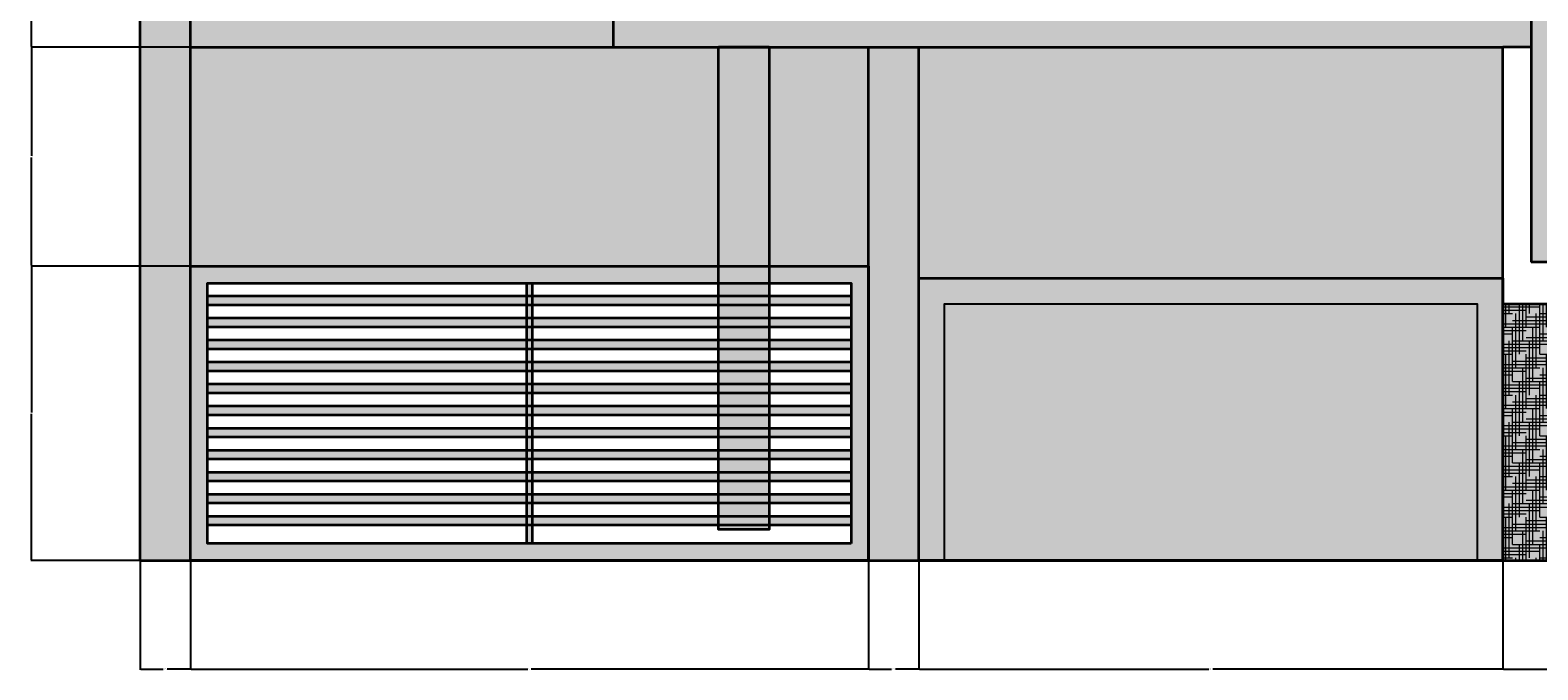
# Model space of a CAD drawing. Units: feet. Extents: x 2415 to 6174, y 866 to 1295.
# Tile 1 of 9: x 3227 to 3580, y 866 to 1016. Entities that reach past the tile are written whole.
import ezdxf

# ---------------------------------------------------------------- set-up
doc = ezdxf.new("R2010")
doc.units = ezdxf.units.FT
for name, color, linetype, lineweight in [('A-ANNO-DIMS', 2, 'Continuous', 18), ('A-DOOR', 4, 'Continuous', 25), ('A-ELEV', 7, 'Continuous', 35), ('A-ELEV-PATT', 8, 'Continuous', 13)]:
    doc.layers.add(name, color=color, linetype=linetype, lineweight=lineweight)
doc.styles.get("Standard").update_dxf_attribs({"font": 'arial.ttf'})
doc.dimstyles.get("Standard").update_dxf_attribs({"dimtxt": 0.18, "dimasz": 0.18, "dimexe": 0.18, "dimexo": 0.0625, "dimgap": 0.09, "dimtad": 0, "dimtih": 1, "dimtoh": 1, "dimdec": 1, "dimzin": 0, "dimdsep": 46, "dimlunit": 3, "dimtxsty": 'Standard', "dimcen": 0.09, "dimadec": 0, "dimazin": 0, "dimtfac": 1, "dimtdec": 1, "dimtofl": 0, "dimtmove": 0, "dimatfit": 3, "dimfxl": 1, "dimtolj": 1, "dimtzin": 0, "dimarcsym": 0})

# ---------------------------------------------------------------- blocks, each defined once
blk = doc.blocks.new('GATE-MAIN')
blk.add_line((0, 60), (124.63, 60))
for points in [[(0, 0), (0, 60)], [(124.63, 60), (124.63, 0)]]:
    blk.add_lwpolyline(points)
blk.add_lwpolyline([(124.63, 0), (0, 0), (0, 60), (124.63, 60)], close=True)
blk = doc.blocks.new('*D53')
at = {"layer": 'A-ANNO-DIMS', "color": 0, "lineweight": -2, "transparency": 16777216}
for p, q in [((3253.13, 891.54), (3253.13, 866.02)), ((3264.92, 891.54), (3264.92, 866.02)), ((3253.31, 866.2), (3258.57, 866.2)), ((3264.74, 866.2), (3259.48, 866.2))]:
    blk.add_line(p, q, dxfattribs=at)
at = {"layer": 'A-ANNO-DIMS', "color": 0, "transparency": 16777216}
for points in [[(3253.31, 866.23), (3253.31, 866.17), (3253.13, 866.2)], [(3264.74, 866.23), (3264.74, 866.17), (3264.92, 866.2)]]:
    blk.add_solid(points, dxfattribs=at)
at = {"layer": 'Defpoints', "color": 0, "transparency": 16777216}
for p in [(3253.13, 891.6), (3264.92, 891.6), (3264.92, 866.2)]:
    blk.add_point(p, dxfattribs=at)
at = {"layer": 'A-ANNO-DIMS', "color": 0, "transparency": 16777216, "insert": (3259.02, 866.2), "char_height": 0.18, "attachment_point": 5}
blk.add_mtext('\\A1;11.787', dxfattribs=at)
blk = doc.blocks.new('*D54')
at = {"layer": 'A-ANNO-DIMS', "color": 0, "lineweight": -2, "transparency": 16777216}
for p, q in [((3264.92, 891.54), (3264.92, 866.02)), ((3423.52, 891.54), (3423.52, 866.02)), ((3265.1, 866.2), (3343.83, 866.2)), ((3423.34, 866.2), (3344.6, 866.2))]:
    blk.add_line(p, q, dxfattribs=at)
at = {"layer": 'A-ANNO-DIMS', "color": 0, "transparency": 16777216}
for points in [[(3265.1, 866.23), (3265.1, 866.17), (3264.92, 866.2)], [(3423.34, 866.23), (3423.34, 866.17), (3423.52, 866.2)]]:
    blk.add_solid(points, dxfattribs=at)
at = {"layer": 'Defpoints', "color": 0, "transparency": 16777216}
for p in [(3264.92, 891.6), (3423.52, 891.6), (3423.52, 866.2)]:
    blk.add_point(p, dxfattribs=at)
at = {"layer": 'A-ANNO-DIMS', "color": 0, "transparency": 16777216, "insert": (3344.22, 866.2), "char_height": 0.18, "attachment_point": 5}
blk.add_mtext('\\A1;158.6', dxfattribs=at)
blk = doc.blocks.new('*D55')
at = {"layer": 'A-ANNO-DIMS', "color": 0, "lineweight": -2, "transparency": 16777216}
for p, q in [((3423.52, 891.54), (3423.52, 866.02)), ((3435.31, 891.54), (3435.31, 866.02)), ((3423.7, 866.2), (3428.96, 866.2)), ((3435.13, 866.2), (3429.87, 866.2))]:
    blk.add_line(p, q, dxfattribs=at)
at = {"layer": 'A-ANNO-DIMS', "color": 0, "transparency": 16777216}
for points in [[(3423.7, 866.23), (3423.7, 866.17), (3423.52, 866.2)], [(3435.13, 866.23), (3435.13, 866.17), (3435.31, 866.2)]]:
    blk.add_solid(points, dxfattribs=at)
at = {"layer": 'Defpoints', "color": 0, "transparency": 16777216}
for p in [(3423.52, 891.6), (3435.31, 891.6), (3435.31, 866.2)]:
    blk.add_point(p, dxfattribs=at)
at = {"layer": 'A-ANNO-DIMS', "color": 0, "transparency": 16777216, "insert": (3429.41, 866.2), "char_height": 0.18, "attachment_point": 5}
blk.add_mtext('\\A1;11.787', dxfattribs=at)
blk = doc.blocks.new('*D56')
at = {"layer": 'A-ANNO-DIMS', "color": 0, "lineweight": -2, "transparency": 16777216}
for p, q in [((3435.31, 891.54), (3435.31, 866.02)), ((3571.93, 891.54), (3571.93, 866.02)), ((3435.49, 866.2), (3503.17, 866.2)), ((3571.75, 866.2), (3504.08, 866.2))]:
    blk.add_line(p, q, dxfattribs=at)
at = {"layer": 'A-ANNO-DIMS', "color": 0, "transparency": 16777216}
for points in [[(3435.49, 866.23), (3435.49, 866.17), (3435.31, 866.2)], [(3571.75, 866.23), (3571.75, 866.17), (3571.93, 866.2)]]:
    blk.add_solid(points, dxfattribs=at)
at = {"layer": 'Defpoints', "color": 0, "transparency": 16777216}
for p in [(3435.31, 891.6), (3571.93, 891.6), (3571.93, 866.2)]:
    blk.add_point(p, dxfattribs=at)
at = {"layer": 'A-ANNO-DIMS', "color": 0, "transparency": 16777216, "insert": (3503.62, 866.2), "char_height": 0.18, "attachment_point": 5}
blk.add_mtext('\\A1;136.63', dxfattribs=at)
blk = doc.blocks.new('*D57')
at = {"layer": 'A-ANNO-DIMS', "color": 0, "lineweight": -2, "transparency": 16777216}
for p, q in [((3571.93, 891.54), (3571.93, 866.02)), ((3601, 891.54), (3601, 866.02)), ((3572.11, 866.2), (3586.07, 866.2)), ((3600.82, 866.2), (3586.86, 866.2))]:
    blk.add_line(p, q, dxfattribs=at)
at = {"layer": 'A-ANNO-DIMS', "color": 0, "transparency": 16777216}
for points in [[(3572.11, 866.23), (3572.11, 866.17), (3571.93, 866.2)], [(3600.82, 866.23), (3600.82, 866.17), (3601, 866.2)]]:
    blk.add_solid(points, dxfattribs=at)
at = {"layer": 'Defpoints', "color": 0, "transparency": 16777216}
for p in [(3571.93, 891.6), (3601, 891.6), (3601, 866.2)]:
    blk.add_point(p, dxfattribs=at)
at = {"layer": 'A-ANNO-DIMS', "color": 0, "transparency": 16777216, "insert": (3586.47, 866.2), "char_height": 0.18, "attachment_point": 5}
blk.add_mtext('\\A1;29.06', dxfattribs=at)
blk = doc.blocks.new('*D72')
at = {"layer": 'A-ANNO-DIMS', "color": 0, "lineweight": -2, "transparency": 16777216}
for p, q in [((3264.85, 960.43), (3227.55, 960.43)), ((3227.73, 960.25), (3227.73, 926.2)), ((3227.73, 891.78), (3227.73, 925.83)), ((3264.85, 891.6), (3227.55, 891.6))]:
    blk.add_line(p, q, dxfattribs=at)
at = {"layer": 'A-ANNO-DIMS', "color": 0, "transparency": 16777216}
for points in [[(3227.7, 960.25), (3227.76, 960.25), (3227.73, 960.43)], [(3227.7, 891.78), (3227.76, 891.78), (3227.73, 891.6)]]:
    blk.add_solid(points, dxfattribs=at)
at = {"layer": 'Defpoints', "color": 0, "transparency": 16777216}
for p in [(3227.73, 960.43), (3264.92, 960.43), (3264.92, 891.6)]:
    blk.add_point(p, dxfattribs=at)
at = {"layer": 'A-ANNO-DIMS', "color": 0, "transparency": 16777216, "insert": (3227.73, 926.02), "char_height": 0.18, "attachment_point": 5}
blk.add_mtext('\\A1;68.83', dxfattribs=at)
blk = doc.blocks.new('*D73')
at = {"layer": 'A-ANNO-DIMS', "color": 0, "lineweight": -2, "transparency": 16777216}
for p, q in [((3264.85, 1011.6), (3227.55, 1011.6)), ((3227.73, 1011.42), (3227.73, 986.2)), ((3227.73, 960.61), (3227.73, 985.83)), ((3264.85, 960.43), (3227.55, 960.43))]:
    blk.add_line(p, q, dxfattribs=at)
at = {"layer": 'A-ANNO-DIMS', "color": 0, "transparency": 16777216}
for points in [[(3227.7, 1011.42), (3227.76, 1011.42), (3227.73, 1011.6)], [(3227.7, 960.61), (3227.76, 960.61), (3227.73, 960.43)]]:
    blk.add_solid(points, dxfattribs=at)
at = {"layer": 'Defpoints', "color": 0, "transparency": 16777216}
for p in [(3227.73, 1011.6), (3264.92, 1011.6), (3264.92, 960.43)]:
    blk.add_point(p, dxfattribs=at)
at = {"layer": 'A-ANNO-DIMS', "color": 0, "transparency": 16777216, "insert": (3227.73, 986.02), "char_height": 0.18, "attachment_point": 5}
blk.add_mtext('\\A1;51.17', dxfattribs=at)
blk = doc.blocks.new('*D74')
at = {"layer": 'A-ANNO-DIMS', "color": 0, "lineweight": -2, "transparency": 16777216}
for p, q in [((3288.28, 1042.32), (3227.55, 1042.32)), ((3227.73, 1042.14), (3227.73, 1027.14)), ((3227.73, 1011.78), (3227.73, 1026.78)), ((3264.85, 1011.6), (3227.55, 1011.6))]:
    blk.add_line(p, q, dxfattribs=at)
at = {"layer": 'A-ANNO-DIMS', "color": 0, "transparency": 16777216}
for points in [[(3227.7, 1042.14), (3227.76, 1042.14), (3227.73, 1042.32)], [(3227.7, 1011.78), (3227.76, 1011.78), (3227.73, 1011.6)]]:
    blk.add_solid(points, dxfattribs=at)
at = {"layer": 'Defpoints', "color": 0, "transparency": 16777216}
for p in [(3227.73, 1042.32), (3288.35, 1042.32), (3264.92, 1011.6)]:
    blk.add_point(p, dxfattribs=at)
at = {"layer": 'A-ANNO-DIMS', "color": 0, "transparency": 16777216, "insert": (3227.73, 1026.96), "char_height": 0.18, "attachment_point": 5}
blk.add_mtext('\\A1;30.72', dxfattribs=at)

msp = doc.modelspace()

# ---------------------------------------------------------------- hatches: boundary and pattern name
at = {"layer": 'A-ELEV-PATT'}
h = msp.add_hatch(color=256, dxfattribs=at)
h.set_gradient(color1=(255, 255, 255), tint=1)
h.paths.add_polyline_path([(3264.916, 1143.5993), (3253.129, 1143.5993), (3253.129, 891.5992), (3264.916, 891.5992)])
h.paths.add_polyline_path([(3470.0448, 1143.5993), (3264.916, 1143.5993), (3264.916, 1137.5993), (3466.5999, 1137.5993)])
h.paths.add_polyline_path([(3363.8667, 1137.5993), (3264.916, 1137.5993), (3264.916, 1011.5992), (3363.8667, 1011.5992)])
h.paths.add_polyline_path([(3286.0429, 1117.0591), (3337.7904, 1117.0591), (3337.7904, 1115.4381), (3336.5314, 1115.4381), (3336.5314, 1110.528), (3335.4882, 1110.528), (3335.4882, 1042.3194), (3288.3452, 1042.3194), (3288.3452, 1110.528), (3287.3019, 1110.528), (3287.3019, 1115.4381), (3286.0429, 1115.4381)], flags=16)
h.paths.add_polyline_path([(3290.3452, 1108.528), (3333.4882, 1108.528), (3333.4882, 1044.3194), (3290.3452, 1044.3194)], flags=0)
h.paths.add_polyline_path([(3292.3452, 1106.528), (3331.4882, 1106.528), (3331.4882, 1046.3194), (3292.3452, 1046.3194)], flags=0)
h.paths.add_polyline_path([(3311.7156, 1106.528), (3312.1178, 1106.528), (3312.1178, 1046.3194), (3311.7156, 1046.3194)], flags=0)
h.paths.add_polyline_path([(3682.0722, 1263.5993), (3578.5579, 1263.5993), (3578.5579, 1137.5993), (3578.5579, 961.3655), (3682.0722, 961.3655)])
h.paths.add_polyline_path([(3660.8129, 1239.0671), (3660.8129, 996.6447), (3602.2151, 996.6447), (3602.2151, 1239.0671)], flags=16)
h.paths.add_polyline_path([(3632.2447, 1239.0671), (3632.2447, 996.6447), (3630.7833, 996.6447), (3630.7833, 1029.3019), (3602.2151, 1029.3019), (3602.2151, 1030.7632), (3630.7833, 1030.7632), (3630.7833, 1071.2549), (3602.2151, 1071.2549), (3602.2151, 1072.7163), (3630.7833, 1072.7163), (3630.7833, 1113.2079), (3602.2151, 1113.2079), (3602.2151, 1114.6693), (3630.7833, 1114.6693), (3630.7833, 1155.161), (3602.2151, 1155.161), (3602.2151, 1156.6224), (3630.7833, 1156.6224), (3630.7833, 1197.114), (3602.2151, 1197.114), (3602.2151, 1198.5754), (3630.7833, 1198.5754), (3630.7833, 1239.0671)], flags=0)
h.paths.add_polyline_path([(3733.129, 951.5993), (3634.5374, 951.5993), (3634.5374, 891.5992), (3733.129, 891.5992)])
h.paths.add_polyline_path([(3627.8799, 951.5993), (3621.0953, 951.5993), (3621.0953, 891.5992), (3627.8799, 891.5992)])
h.paths.add_polyline_path([(3614.4378, 951.5993), (3607.6532, 951.5993), (3607.6532, 891.5992), (3614.4378, 891.5992)])
h.paths.add_polyline_path([(3565.9347, 951.5993), (3441.3079, 951.5993), (3441.3079, 891.5992), (3565.9347, 891.5992)], flags=17)
h.paths.add_polyline_path([(3571.9347, 957.5993), (3435.3079, 957.5993), (3435.3079, 891.5992), (3441.3079, 891.5992), (3441.3079, 951.5993), (3565.9347, 951.5993), (3565.9347, 891.5992), (3571.9347, 891.5992)])
h.paths.add_polyline_path([(3435.3079, 1011.5992), (3423.5209, 1011.5992), (3423.5209, 891.5992), (3435.3079, 891.5992), (3435.3079, 957.5993)])
h.paths.add_polyline_path([(3690.0912, 1269.5993), (3571.9347, 1269.5993), (3571.9347, 1263.5993), (3690.0912, 1263.5993)])
h.paths.add_polyline_path([(3571.9347, 1269.5993), (3538.5122, 1257.6449), (3538.5122, 1251.6449), (3571.9347, 1263.5993)])
h = msp.add_hatch(color=256, dxfattribs=at)
h.set_gradient(color1=(99, 100, 102), color2=(99, 100, 102))
h.paths.add_polyline_path([(3578.5579, 1137.5993), (3363.8667, 1137.5993), (3363.8667, 1123.5993), (3371.8667, 1123.5993), (3371.8667, 1129.5993), (3570.5579, 1129.5993), (3570.5579, 1019.5993), (3371.8667, 1019.5993), (3371.8667, 1027.963), (3363.8667, 1027.963), (3363.8667, 1011.5992), (3571.9347, 1011.5992), (3578.5579, 1011.5992)])
h.paths.add_polyline_path([(3371.8667, 1123.5993), (3363.8667, 1123.5993), (3363.8667, 1053.4585), (3371.8667, 1053.4585)], flags=17)
h.paths.add_polyline_path([(3371.8667, 1042.1234), (3363.8667, 1042.1234), (3363.8667, 1028.2269), (3371.8667, 1028.2269)], flags=17)
h.paths.add_polyline_path([(3371.8667, 1051.7117), (3363.8667, 1051.7117), (3363.8667, 1042.3873), (3371.8667, 1042.3873)], flags=17)
h.paths.add_polyline_path([(3371.8667, 1053.4585), (3363.8667, 1053.4585), (3363.8667, 1051.7117), (3371.8667, 1051.7117)], flags=17)
h.paths.add_polyline_path([(3371.8667, 1042.3873), (3363.8667, 1042.3873), (3363.8667, 1042.1234), (3371.8667, 1042.1234)], flags=17)
h.paths.add_polyline_path([(3371.8667, 1028.2269), (3363.8667, 1028.2269), (3363.8667, 1027.963), (3371.8667, 1027.963)], flags=17)
h = msp.add_hatch(color=256, dxfattribs=at)
h.set_gradient(color1=(248, 246, 176), name='CURVED')
h.paths.add_polyline_path([(3487.443, 1123.5993), (3446.1534, 1123.5993), (3446.1534, 1053.4585), (3487.443, 1053.4585), (3487.443, 1080.8275)])
h.paths.add_polyline_path([(3468.3641, 1051.7117), (3446.1534, 1051.7117), (3446.1534, 1028.2269), (3468.3641, 1028.2269)])
h.paths.add_polyline_path([(3487.443, 1051.7117), (3468.628, 1051.7117), (3468.628, 1028.2269), (3487.443, 1028.2269)])
h.paths.add_polyline_path([(3468.3641, 1027.963), (3446.1534, 1027.963), (3446.1534, 1019.5993), (3468.3641, 1019.5993)])
h.paths.add_polyline_path([(3487.443, 1027.963), (3468.628, 1027.963), (3468.628, 1019.5993), (3487.443, 1019.5993)])
h.paths.add_polyline_path([(3564.5579, 1123.5993), (3530.9457, 1099.6515), (3487.443, 1099.6515), (3487.443, 1080.8275), (3524.8012, 1080.8275), (3524.8012, 1053.4585), (3564.5579, 1053.4585)])
h.paths.add_polyline_path([(3548.7638, 1051.7117), (3524.8012, 1051.7117), (3524.8012, 1028.2269), (3548.7638, 1028.2269)])
h.paths.add_polyline_path([(3548.7638, 1027.963), (3524.8012, 1027.963), (3524.8012, 1019.5993), (3548.7638, 1019.5993)])
h.paths.add_polyline_path([(3564.5579, 1027.963), (3549.0277, 1027.963), (3549.0277, 1019.5993), (3564.5579, 1019.5993)])
h.paths.add_polyline_path([(3388.4421, 1011.5992), (3264.916, 1011.5992), (3264.916, 960.433), (3388.4421, 960.433)])
h.paths.add_polyline_path([(3571.9347, 1011.5992), (3435.3079, 1011.5992), (3435.3079, 957.5993), (3571.9347, 957.5993)])
h.paths.add_polyline_path([(3423.5209, 1011.5992), (3400.3333, 1011.5992), (3400.3333, 960.433), (3423.5209, 960.433)])
h = msp.add_hatch(color=256, dxfattribs=at)
h.set_gradient(color1=(203, 74, 40), color2=(203, 74, 40))
h.paths.add_polyline_path([(3400.3333, 1011.5992), (3388.4421, 1011.5992), (3388.4421, 960.433), (3400.3333, 960.433)])
h.paths.add_polyline_path([(3400.3333, 956.433), (3388.4421, 956.433), (3388.4421, 953.4503), (3400.3333, 953.4503)])
h.paths.add_polyline_path([(3400.3333, 951.2861), (3388.4421, 951.2861), (3388.4421, 948.3033), (3400.3333, 948.3033)])
h.paths.add_polyline_path([(3400.3333, 946.1391), (3388.4421, 946.1391), (3388.4421, 943.1563), (3400.3333, 943.1563)])
h.paths.add_polyline_path([(3400.3333, 940.9922), (3388.4421, 940.9922), (3388.4421, 938.0094), (3400.3333, 938.0094)])
h.paths.add_polyline_path([(3400.3333, 935.8452), (3388.4421, 935.8452), (3388.4421, 932.8624), (3400.3333, 932.8624)])
h.paths.add_polyline_path([(3400.3333, 930.6983), (3388.4421, 930.6983), (3388.4421, 927.7155), (3400.3333, 927.7155)])
h.paths.add_polyline_path([(3400.3333, 925.5513), (3388.4421, 925.5513), (3388.4421, 922.5685), (3400.3333, 922.5685)])
h.paths.add_polyline_path([(3400.3333, 920.4043), (3388.4421, 920.4043), (3388.4421, 917.4215), (3400.3333, 917.4215)])
h.paths.add_polyline_path([(3400.3333, 915.2574), (3388.4421, 915.2574), (3388.4421, 912.2746), (3400.3333, 912.2746)])
h.paths.add_polyline_path([(3400.3333, 910.1104), (3388.4421, 910.1104), (3388.4421, 907.1276), (3400.3333, 907.1276)])
h.paths.add_polyline_path([(3400.3333, 904.9635), (3388.4421, 904.9635), (3388.4421, 901.9807), (3400.3333, 901.9807)])
h.paths.add_polyline_path([(3400.3333, 899.8165), (3388.4421, 899.8165), (3388.4421, 898.815), (3400.3333, 898.815)])
h = msp.add_hatch(color=256, dxfattribs=at)
h.set_gradient(color1=(248, 246, 176), color2=(248, 246, 176), name='CURVED')
h.paths.add_polyline_path([(3571.9347, 1011.5992), (3435.3079, 1011.5992), (3435.3079, 957.5993), (3571.9347, 957.5993)])
h = msp.add_hatch(color=256, dxfattribs=at)
h.set_gradient(color1=(147, 149, 152), color2=(99, 100, 102))
h.paths.add_polyline_path([(3423.523, 960.4469), (3264.9181, 960.4469), (3264.9181, 891.6131), (3423.523, 891.6131)])
h.paths.add_polyline_path([(3268.9181, 956.4469), (3419.523, 956.4469), (3419.523, 895.6131), (3268.9181, 895.6131)], flags=16)
h.paths.add_polyline_path([(3268.9181, 953.4641), (3343.5898, 953.4641), (3343.5898, 956.4469), (3344.8513, 956.4469), (3344.8513, 953.4641), (3419.523, 953.4641), (3419.523, 951.2999), (3344.8513, 951.2999), (3344.8513, 948.3172), (3419.523, 948.3172), (3419.523, 946.153), (3344.8513, 946.153), (3344.8513, 943.1702), (3419.523, 943.1702), (3419.523, 941.006), (3344.8513, 941.006), (3344.8513, 938.0232), (3419.523, 938.0232), (3419.523, 935.8591), (3344.8513, 935.8591), (3344.8513, 932.8763), (3419.523, 932.8763), (3419.523, 930.7121), (3344.8513, 930.7121), (3344.8513, 927.7293), (3419.523, 927.7293), (3419.523, 925.5652), (3344.8513, 925.5652), (3344.8513, 922.5824), (3419.523, 922.5824), (3419.523, 920.4182), (3344.8513, 920.4182), (3344.8513, 917.4354), (3419.523, 917.4354), (3419.523, 915.2712), (3344.8513, 915.2712), (3344.8513, 912.2884), (3419.523, 912.2884), (3419.523, 910.1243), (3344.8513, 910.1243), (3344.8513, 907.1415), (3419.523, 907.1415), (3419.523, 904.9773), (3344.8513, 904.9773), (3344.8513, 901.9945), (3419.523, 901.9945), (3419.523, 899.8304), (3344.8513, 899.8304), (3344.8513, 895.6131), (3343.5898, 895.6131), (3343.5898, 899.8304), (3268.9181, 899.8304), (3268.9181, 901.9945), (3343.5898, 901.9945), (3343.5898, 904.9773), (3268.9181, 904.9773), (3268.9181, 907.1415), (3343.5898, 907.1415), (3343.5898, 910.1243), (3268.9181, 910.1243), (3268.9181, 912.2884), (3343.5898, 912.2884), (3343.5898, 915.2712), (3268.9181, 915.2712), (3268.9181, 917.4354), (3343.5898, 917.4354), (3343.5898, 920.4182), (3268.9181, 920.4182), (3268.9181, 922.5824), (3343.5898, 922.5824), (3343.5898, 925.5652), (3268.9181, 925.5652), (3268.9181, 927.7293), (3343.5898, 927.7293), (3343.5898, 930.7121), (3268.9181, 930.7121), (3268.9181, 932.8763), (3343.5898, 932.8763), (3343.5898, 935.8591), (3268.9181, 935.8591), (3268.9181, 938.0232), (3343.5898, 938.0232), (3343.5898, 941.006), (3268.9181, 941.006), (3268.9181, 943.1702), (3343.5898, 943.1702), (3343.5898, 946.153), (3268.9181, 946.153), (3268.9181, 948.3172), (3343.5898, 948.3172), (3343.5898, 951.2999), (3268.9181, 951.2999)], flags=16)
h = msp.add_hatch(color=256, dxfattribs=at)
h.set_gradient(color1=(99, 100, 102), color2=(99, 100, 102))
h.paths.add_polyline_path([(3607.6532, 957.5993), (3600.9957, 957.5993), (3600.9957, 891.5992), (3607.6532, 891.5992)])
h.paths.add_polyline_path([(3621.0953, 957.5993), (3614.4378, 957.5993), (3614.4378, 891.5992), (3621.0953, 891.5992)])
h.paths.add_polyline_path([(3634.5374, 957.5993), (3627.8799, 957.5993), (3627.8799, 891.5992), (3634.5374, 891.5992)])
h.paths.add_polyline_path([(3600.9957, 951.5993), (3571.9347, 951.5993), (3571.9347, 891.5992), (3600.9957, 891.5992)])
h = msp.add_hatch(dxfattribs=at)
h.set_pattern_fill('HOUND', color=256, scale=0.5, style=0)
h.set_pattern_definition([(0, (850.0754, 0), (3.175, 0.79375), [12.7, -6.35]), (90, (850.0754, 0), (-0.79375, -3.175), [12.7, -6.35])])
h.paths.add_polyline_path([(3607.6532, 957.5993), (3600.9957, 957.5993), (3600.9957, 891.5992), (3607.6532, 891.5992)])
h.paths.add_polyline_path([(3621.0953, 957.5993), (3614.4378, 957.5993), (3614.4378, 891.5992), (3621.0953, 891.5992)])
h.paths.add_polyline_path([(3634.5374, 957.5993), (3627.8799, 957.5993), (3627.8799, 891.5992), (3634.5374, 891.5992)])
h.paths.add_polyline_path([(3600.9957, 951.5993), (3571.9347, 951.5993), (3571.9347, 891.5992), (3600.9957, 891.5992)])

# ---------------------------------------------------------------- linework, layer by layer
at = {"layer": 'A-ELEV'}
for p, q in [((3253.129, 891.5992), (3253.129, 1143.5993)), ((3363.8667, 1011.5992), (3363.8667, 1137.5993)), ((3578.5579, 1137.5993), (3578.5579, 961.3655)), ((3264.916, 1011.5992), (3571.9347, 1011.5992)), ((3423.5209, 891.5992), (3423.5209, 1011.5992)), ((3435.3079, 891.5992), (3435.3079, 1011.5992)), ((3571.9347, 891.5992), (3571.9347, 1011.5992)), ((3435.3079, 957.5993), (3571.9347, 957.5993)), ((3571.9347, 951.5993), (3600.9957, 951.5993)), ((3253.129, 891.5992), (3733.129, 891.5992))]:
    msp.add_line(p, q, dxfattribs=at)
for points in [[(3682.0722, 1263.5993), (3682.0722, 961.3655), (3578.5579, 961.3655)], [(3253.129, 891.5992), (3264.916, 891.5992), (3264.916, 1143.5993)], [(3578.5579, 1137.5993), (3578.5579, 1137.5993), (3578.5579, 1011.5992), (3571.9347, 1011.5992)], [(3400.3333, 1011.5992), (3388.4421, 1011.5992)], [(3400.3333, 1011.5992), (3400.3333, 898.815), (3388.4421, 898.815), (3388.4421, 1011.5992)], [(3423.5209, 891.5992), (3435.3079, 891.5992)], [(3571.9347, 891.5992), (3435.3079, 891.5992)]]:
    msp.add_lwpolyline(points, dxfattribs=at)
for points in [[(3423.5209, 891.5992), (3264.916, 891.5992), (3264.916, 960.433), (3423.5209, 960.433)], [(3419.5209, 895.5993), (3268.916, 895.5993), (3268.916, 956.433), (3419.5209, 956.433)], [(3343.5877, 956.433), (3344.8492, 956.433), (3344.8492, 895.5993), (3343.5877, 895.5993)], [(3571.9347, 891.5992), (3435.3079, 891.5992), (3435.3079, 957.5993), (3571.9347, 957.5993)], [(3268.916, 953.4503), (3419.5209, 953.4503), (3419.5209, 951.2861), (3268.916, 951.2861)], [(3268.916, 948.3033), (3419.5209, 948.3033), (3419.5209, 946.1391), (3268.916, 946.1391)], [(3268.916, 943.1563), (3419.5209, 943.1563), (3419.5209, 940.9922), (3268.916, 940.9922)], [(3268.916, 938.0094), (3419.5209, 938.0094), (3419.5209, 935.8452), (3268.916, 935.8452)], [(3268.916, 932.8624), (3419.5209, 932.8624), (3419.5209, 930.6983), (3268.916, 930.6983)], [(3268.916, 927.7155), (3419.5209, 927.7155), (3419.5209, 925.5513), (3268.916, 925.5513)], [(3268.916, 922.5685), (3419.5209, 922.5685), (3419.5209, 920.4043), (3268.916, 920.4043)], [(3268.916, 917.4215), (3419.5209, 917.4215), (3419.5209, 915.2574), (3268.916, 915.2574)], [(3268.916, 912.2746), (3419.5209, 912.2746), (3419.5209, 910.1104), (3268.916, 910.1104)], [(3268.916, 907.1276), (3419.5209, 907.1276), (3419.5209, 904.9635), (3268.916, 904.9635)], [(3268.916, 901.9807), (3419.5209, 901.9807), (3419.5209, 899.8165), (3268.916, 899.8165)]]:
    msp.add_lwpolyline(points, close=True, dxfattribs=at)

# ---------------------------------------------------------------- block references
at = {"layer": 'A-DOOR'}
msp.add_blockref('GATE-MAIN', (3441.308, 891.599), dxfattribs=at)

# ---------------------------------------------------------------- dimensions: what is measured, and where the dimension line sits
at = {"layer": 'A-ANNO-DIMS'}
for base, p1, p2, picture, middle in [((3227.729, 1042.3194), (3264.916, 1011.5992), (3288.3452, 1042.3194), '*D74', (3227.729, 1026.9593)), ((3227.729, 1011.5992), (3264.916, 960.433), (3264.916, 1011.5992), '*D73', (3227.729, 986.0161)), ((3227.729, 960.433), (3264.916, 891.5992), (3264.916, 960.433), '*D72', (3227.729, 926.0161))]:
    dim = msp.add_linear_dim(base=base, p1=p1, p2=p2, angle=90, dimstyle='Standard', override={"dimdec": 2, "dimlfac": 1, "dimrnd": 0, "dimzin": 0, "dimdsep": 46, "dimlunit": 2}, dxfattribs=at)
    dim.commit()
    dim.dimension.update_dxf_attribs({"geometry": picture, "text_midpoint": middle})
for base, p1, p2, override, picture, middle in [((3264.916, 866.1993), (3253.129, 891.5992), (3264.916, 891.5992), {"dimdec": 3, "dimlfac": 1, "dimrnd": 0, "dimzin": 0, "dimdsep": 46, "dimlunit": 2}, '*D53', (3259.0225, 866.1993)), ((3423.5209, 866.1993), (3264.916, 891.5992), (3423.5209, 891.5992), {"dimdec": 1, "dimlfac": 1, "dimrnd": 0, "dimzin": 0, "dimdsep": 46, "dimlunit": 2}, '*D54', (3344.2184, 866.1993)), ((3435.3079, 866.1993), (3423.5209, 891.5992), (3435.3079, 891.5992), {"dimdec": 3, "dimlfac": 1, "dimrnd": 0, "dimzin": 0, "dimdsep": 46, "dimlunit": 2}, '*D55', (3429.4144, 866.1993)), ((3571.9347, 866.1993), (3435.3079, 891.5992), (3571.9347, 891.5992), {"dimdec": 2, "dimlfac": 1, "dimrnd": 0, "dimzin": 0, "dimdsep": 46, "dimlunit": 2}, '*D56', (3503.6213, 866.1993)), ((3600.9957, 866.1993), (3571.9347, 891.5992), (3600.9957, 891.5992), {"dimdec": 2, "dimlfac": 1, "dimrnd": 0, "dimzin": 0, "dimdsep": 46, "dimlunit": 2}, '*D57', (3586.4652, 866.1993))]:
    dim = msp.add_linear_dim(base=base, p1=p1, p2=p2, dimstyle='Standard', override=override, dxfattribs=at)
    dim.commit()
    dim.dimension.update_dxf_attribs({"geometry": picture, "text_midpoint": middle})

doc.saveas('drawing.dxf')
